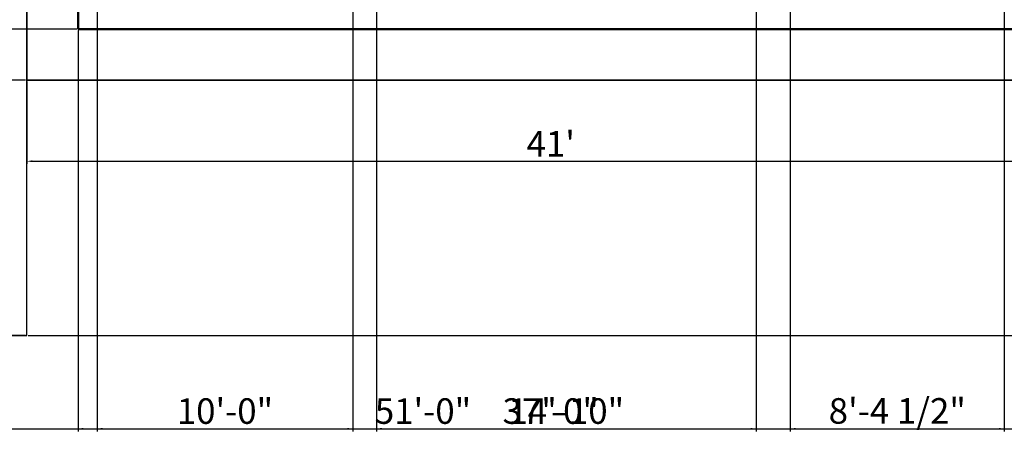
# Model space of a CAD drawing. Units: inches. Extents: x 5307 to 6359, y 4763 to 5474.
# Tile 2 of 5: x 5543 to 6006, y 4763 to 4966. Entities that reach past the tile are written whole.
import ezdxf

# ---------------------------------------------------------------- set-up
doc = ezdxf.new("R2010")
doc.units = ezdxf.units.IN
for name, color, linetype, lineweight in [('A-ANNO-DIMS', 2, 'Continuous', 18), ('A-WALL', 7, 'Continuous', 50), ('C-PROP', 7, 'Continuous', 35), ('ROAD', 240, 'Continuous', 25)]:
    doc.layers.add(name, color=color, linetype=linetype, lineweight=lineweight)
doc.styles.get("Standard").update_dxf_attribs({"font": 'arial.ttf'})
doc.dimstyles.new('ISO-25', dxfattribs={"dimtxt": 12, "dimasz": 2.5, "dimexe": 1.25, "dimexo": 0.625, "dimtad": 1, "dimtih": 1, "dimtoh": 1, "dimlunit": 4, "dimtxsty": 'Standard', "dimcen": 2.5, "dimadec": 0, "dimazin": 0, "dimtfac": 1, "dimtmove": 0, "dimatfit": 3, "dimfxl": 1, "dimarcsym": 0})

# ---------------------------------------------------------------- blocks, each defined once
blk = doc.blocks.new('*D3')
at = {"layer": 'A-ANNO-DIMS', "color": 0, "lineweight": -2, "transparency": 16777216}
for p, q in [((5545.97, 5237.78), (5511.45, 5237.78)), ((5512.7, 5235.28), (5512.7, 5094.54)), ((5512.7, 4940.28), (5512.7, 5081.03)), ((5545.97, 4937.78), (5511.45, 4937.78))]:
    blk.add_line(p, q, dxfattribs=at)
at = {"layer": 'A-ANNO-DIMS', "color": 0, "transparency": 16777216}
for points in [[(5512.28, 5235.28), (5513.12, 5235.28), (5512.7, 5237.78)], [(5512.28, 4940.28), (5513.12, 4940.28), (5512.7, 4937.78)]]:
    blk.add_solid(points, dxfattribs=at)
at = {"layer": 'Defpoints', "color": 0, "transparency": 16777216}
for p in [(5546.59, 5237.78), (5512.7, 4937.78), (5546.59, 4937.78)]:
    blk.add_point(p, dxfattribs=at)
at = {"layer": 'A-ANNO-DIMS', "color": 0, "transparency": 16777216, "insert": (5512.7, 5087.78), "char_height": 12, "attachment_point": 5}
blk.add_mtext("25'", dxfattribs=at)
blk = doc.blocks.new('*D4')
at = {"layer": 'A-ANNO-DIMS', "color": 0, "lineweight": -2, "transparency": 16777216}
for p, q in [((5546.59, 4937.16), (5546.59, 4898.47)), ((6038.59, 4937.64), (6038.59, 4898.47)), ((5549.09, 4899.72), (6036.09, 4899.72))]:
    blk.add_line(p, q, dxfattribs=at)
at = {"layer": 'A-ANNO-DIMS', "color": 0, "transparency": 16777216}
for points in [[(5549.09, 4900.14), (5549.09, 4899.3), (5546.59, 4899.72)], [(6036.09, 4900.14), (6036.09, 4899.3), (6038.59, 4899.72)]]:
    blk.add_solid(points, dxfattribs=at)
at = {"layer": 'Defpoints', "color": 0, "transparency": 16777216}
for p in [(6038.59, 4938.26), (5546.59, 4937.78), (6038.59, 4899.72)]:
    blk.add_point(p, dxfattribs=at)
at = {"layer": 'A-ANNO-DIMS', "color": 0, "transparency": 16777216, "insert": (5792.59, 4906.37), "char_height": 12, "attachment_point": 5}
blk.add_mtext("41'", dxfattribs=at)
blk = doc.blocks.new('*D12')
at = {"layer": 'A-ANNO-DIMS', "color": 0, "lineweight": -2, "transparency": 16777216}
for p, q in [((6038.59, 4937.16), (6038.59, 4772.78)), ((5426.59, 4817.16), (5426.59, 4772.78)), ((5429.09, 4774.03), (6036.09, 4774.03))]:
    blk.add_line(p, q, dxfattribs=at)
at = {"layer": 'A-ANNO-DIMS', "color": 0, "transparency": 16777216}
for points in [[(5429.09, 4774.45), (5429.09, 4773.62), (5426.59, 4774.03)], [(6036.09, 4774.45), (6036.09, 4773.62), (6038.59, 4774.03)]]:
    blk.add_solid(points, dxfattribs=at)
at = {"layer": 'Defpoints', "color": 0, "transparency": 16777216}
for p in [(6038.59, 4937.78), (5426.59, 4817.78), (6038.59, 4774.03)]:
    blk.add_point(p, dxfattribs=at)
at = {"layer": 'A-ANNO-DIMS', "color": 0, "transparency": 16777216, "insert": (5732.59, 4780.79), "char_height": 12, "attachment_point": 5}
blk.add_mtext('51\'-0"', dxfattribs=at)
blk = doc.blocks.new('*D13')
at = {"layer": 'A-ANNO-DIMS', "color": 0, "lineweight": -2, "transparency": 16777216}
for p, q in [((6038.88, 5405.78), (6325.25, 5405.78)), ((6324, 5403.28), (6324, 5118.54)), ((6324, 4820.28), (6324, 5105.03)), ((5547.22, 4817.78), (6325.25, 4817.78))]:
    blk.add_line(p, q, dxfattribs=at)
at = {"layer": 'A-ANNO-DIMS', "color": 0, "transparency": 16777216}
for points in [[(6323.58, 5403.28), (6324.41, 5403.28), (6324, 5405.78)], [(6323.58, 4820.28), (6324.41, 4820.28), (6324, 4817.78)]]:
    blk.add_solid(points, dxfattribs=at)
at = {"layer": 'Defpoints', "color": 0, "transparency": 16777216}
for p in [(6038.25, 5405.78), (6324, 5405.78), (5546.59, 4817.78)]:
    blk.add_point(p, dxfattribs=at)
at = {"layer": 'A-ANNO-DIMS', "color": 0, "transparency": 16777216, "insert": (6324, 5111.78), "char_height": 12, "attachment_point": 5}
blk.add_mtext('49\'-0"', dxfattribs=at)
blk = doc.blocks.new('*D15')
at = {"layer": 'A-ANNO-DIMS', "color": 0, "lineweight": -2, "transparency": 16777216}
for p, q in [((5569.97, 4961.78), (5381.59, 4961.78)), ((5382.84, 4959.28), (5382.84, 4956.54)), ((5382.84, 4940.28), (5382.84, 4943.03)), ((5545.97, 4937.78), (5381.59, 4937.78))]:
    blk.add_line(p, q, dxfattribs=at)
at = {"layer": 'A-ANNO-DIMS', "color": 0, "transparency": 16777216}
for points in [[(5382.43, 4959.28), (5383.26, 4959.28), (5382.84, 4961.78)], [(5382.43, 4940.28), (5383.26, 4940.28), (5382.84, 4937.78)]]:
    blk.add_solid(points, dxfattribs=at)
at = {"layer": 'Defpoints', "color": 0, "transparency": 16777216}
for p in [(5382.84, 4961.78), (5570.59, 4961.78), (5546.59, 4937.78)]:
    blk.add_point(p, dxfattribs=at)
at = {"layer": 'A-ANNO-DIMS', "color": 0, "transparency": 16777216, "insert": (5382.84, 4949.78), "char_height": 12, "attachment_point": 5}
blk.add_mtext('2\'-0"', dxfattribs=at)
blk = doc.blocks.new('*D18')
at = {"layer": 'A-ANNO-DIMS', "color": 0, "lineweight": -2, "transparency": 16777216}
for p, q in [((5545.97, 4937.78), (5381.59, 4937.78)), ((5382.84, 4935.28), (5382.84, 4884.54)), ((5382.84, 4820.28), (5382.84, 4871.03)), ((5545.97, 4817.78), (5381.59, 4817.78))]:
    blk.add_line(p, q, dxfattribs=at)
at = {"layer": 'A-ANNO-DIMS', "color": 0, "transparency": 16777216}
for points in [[(5382.43, 4935.28), (5383.26, 4935.28), (5382.84, 4937.78)], [(5382.43, 4820.28), (5383.26, 4820.28), (5382.84, 4817.78)]]:
    blk.add_solid(points, dxfattribs=at)
at = {"layer": 'Defpoints', "color": 0, "transparency": 16777216}
for p in [(5382.84, 4937.78), (5546.59, 4937.78), (5546.59, 4817.78)]:
    blk.add_point(p, dxfattribs=at)
at = {"layer": 'A-ANNO-DIMS', "color": 0, "transparency": 16777216, "insert": (5382.84, 4877.78), "char_height": 12, "attachment_point": 5}
blk.add_mtext('10\'-0"', dxfattribs=at)
blk = doc.blocks.new('*D24')
at = {"layer": 'A-ANNO-DIMS', "color": 0, "lineweight": -2, "transparency": 16777216}
for p, q in [((5579.59, 4970.16), (5579.59, 4772.78)), ((5699.59, 4970.16), (5699.59, 4772.78)), ((5582.09, 4774.03), (5697.09, 4774.03))]:
    blk.add_line(p, q, dxfattribs=at)
at = {"layer": 'A-ANNO-DIMS', "color": 0, "transparency": 16777216}
for points in [[(5582.09, 4774.45), (5582.09, 4773.62), (5579.59, 4774.03)], [(5697.09, 4774.45), (5697.09, 4773.62), (5699.59, 4774.03)]]:
    blk.add_solid(points, dxfattribs=at)
at = {"layer": 'Defpoints', "color": 0, "transparency": 16777216}
for p in [(5579.59, 4970.78), (5699.59, 4970.78), (5699.59, 4774.03)]:
    blk.add_point(p, dxfattribs=at)
at = {"layer": 'A-ANNO-DIMS', "color": 0, "transparency": 16777216, "insert": (5639.59, 4780.79), "char_height": 12, "attachment_point": 5}
blk.add_mtext('10\'-0"', dxfattribs=at)
blk = doc.blocks.new('*D25')
at = {"layer": 'A-ANNO-DIMS', "color": 0, "lineweight": -2, "transparency": 16777216}
for p, q in [((5710.76, 4970.16), (5710.76, 4772.78)), ((5889, 4970.05), (5889, 4772.78)), ((5713.26, 4774.03), (5886.5, 4774.03))]:
    blk.add_line(p, q, dxfattribs=at)
at = {"layer": 'A-ANNO-DIMS', "color": 0, "transparency": 16777216}
for points in [[(5713.26, 4774.45), (5713.26, 4773.62), (5710.76, 4774.03)], [(5886.5, 4774.45), (5886.5, 4773.62), (5889, 4774.03)]]:
    blk.add_solid(points, dxfattribs=at)
at = {"layer": 'Defpoints', "color": 0, "transparency": 16777216}
for p in [(5710.76, 4970.78), (5889, 4970.67), (5889, 4774.03)]:
    blk.add_point(p, dxfattribs=at)
at = {"layer": 'A-ANNO-DIMS', "color": 0, "transparency": 16777216, "insert": (5799.88, 4780.79), "char_height": 12, "attachment_point": 5}
blk.add_mtext('14\'-10"', dxfattribs=at)
blk = doc.blocks.new('*D26')
at = {"layer": 'A-ANNO-DIMS', "color": 0, "lineweight": -2, "transparency": 16777216}
for p, q in [((5905.06, 4970.06), (5905.06, 4772.78)), ((6005.56, 4970.16), (6005.56, 4772.78)), ((5907.56, 4774.03), (6003.06, 4774.03))]:
    blk.add_line(p, q, dxfattribs=at)
at = {"layer": 'A-ANNO-DIMS', "color": 0, "transparency": 16777216}
for points in [[(5907.56, 4774.45), (5907.56, 4773.62), (5905.06, 4774.03)], [(6003.06, 4774.45), (6003.06, 4773.62), (6005.56, 4774.03)]]:
    blk.add_solid(points, dxfattribs=at)
at = {"layer": 'Defpoints', "color": 0, "transparency": 16777216}
for p in [(5905.06, 4970.69), (6005.56, 4970.78), (6005.56, 4774.03)]:
    blk.add_point(p, dxfattribs=at)
at = {"layer": 'A-ANNO-DIMS', "color": 0, "transparency": 16777216, "insert": (5955.31, 4780.86), "char_height": 12, "attachment_point": 5}
blk.add_mtext('8\'-4 1/2"', dxfattribs=at)
blk = doc.blocks.new('*D33')
at = {"layer": 'A-ANNO-DIMS', "color": 0, "lineweight": -2, "transparency": 16777216}
for p, q in [((5570.59, 4961.16), (5570.59, 4772.78)), ((6014.57, 4961.16), (6014.57, 4772.78)), ((5573.09, 4774.03), (6012.07, 4774.03))]:
    blk.add_line(p, q, dxfattribs=at)
at = {"layer": 'A-ANNO-DIMS', "color": 0, "transparency": 16777216}
for points in [[(5573.09, 4774.45), (5573.09, 4773.62), (5570.59, 4774.03)], [(6012.07, 4774.45), (6012.07, 4773.62), (6014.57, 4774.03)]]:
    blk.add_solid(points, dxfattribs=at)
at = {"layer": 'Defpoints', "color": 0, "transparency": 16777216}
for p in [(5570.59, 4961.78), (6014.57, 4961.78), (6014.57, 4774.03)]:
    blk.add_point(p, dxfattribs=at)
at = {"layer": 'A-ANNO-DIMS', "color": 0, "transparency": 16777216, "insert": (5792.58, 4780.79), "char_height": 12, "attachment_point": 5}
blk.add_mtext('37\'-0"', dxfattribs=at)

msp = doc.modelspace()

# ---------------------------------------------------------------- linework, layer by layer
at = {"layer": 'A-WALL'}
for p, q in [((5570.592, 5213.807), (5570.592, 4961.784)), ((5570.592, 4961.784), (6014.569, 4961.784)), ((5881.069, 4961.654), (5881.069, 4961.784)), ((5885.569, 4961.659), (5885.569, 4961.784))]:
    msp.add_line(p, q, dxfattribs=at)
at = {"layer": 'C-PROP'}
for p, q in [((5546.592, 5237.784), (5546.592, 4937.784)), ((5546.592, 4937.784), (6038.592, 4937.784))]:
    msp.add_line(p, q, dxfattribs=at)
at = {"layer": 'ROAD'}
for p, q in [((5546.592, 4817.784), (5546.592, 4937.784)), ((5426.592, 4817.784), (5546.592, 4817.784))]:
    msp.add_line(p, q, dxfattribs=at)

# ---------------------------------------------------------------- dimensions: what is measured, and where the dimension line sits
at = {"layer": 'A-ANNO-DIMS'}
for base, p1, p2, override, picture, middle in [((6323.996, 5405.784), (5546.592, 4817.784), (6038.255, 5405.784), {"dimdec": 1, "dimlfac": 1, "dimrnd": 0, "dimzin": 1, "dimdsep": 46, "dimlunit": 4, "dimfrac": 2}, '*D13', (6323.996, 5111.784)), ((5512.7, 4937.784), (5546.592, 5237.784), (5546.592, 4937.784), {"dimclrd": 0, "dimclre": 0, "dimclrt": 0}, '*D3', (5512.7, 5087.784)), ((5382.842, 4961.784), (5546.592, 4937.784), (5570.592, 4961.784), {"dimdec": 1, "dimlfac": 1, "dimrnd": 0, "dimzin": 1, "dimdsep": 46, "dimlunit": 4, "dimfrac": 2}, '*D15', (5382.842, 4949.784)), ((5382.842, 4937.784), (5546.592, 4817.784), (5546.592, 4937.784), {"dimdec": 1, "dimlfac": 1, "dimrnd": 0, "dimzin": 1, "dimdsep": 46, "dimlunit": 4, "dimfrac": 2}, '*D18', (5382.842, 4877.784))]:
    dim = msp.add_linear_dim(base=base, p1=p1, p2=p2, angle=90, dimstyle='ISO-25', override=override, dxfattribs=at)
    dim.commit()
    dim.dimension.update_dxf_attribs({"geometry": picture, "text_midpoint": middle})
for base, p1, p2, override, picture, middle in [((5699.592, 4774.034), (5579.592, 4970.784), (5699.592, 4970.784), {"dimdec": 1, "dimlfac": 1, "dimrnd": 0, "dimzin": 1, "dimdsep": 46, "dimlunit": 4, "dimfrac": 2}, '*D24', (5639.592, 4780.786)), ((5889.001, 4774.034), (5710.758, 4970.784), (5889.001, 4970.671), {"dimdec": 1, "dimlfac": 1, "dimrnd": 0, "dimzin": 1, "dimdsep": 46, "dimlunit": 4, "dimfrac": 2}, '*D25', (5799.88, 4780.786)), ((6005.56, 4774.034), (5905.06, 4970.686), (6005.56, 4970.784), {"dimdec": 1, "dimlfac": 1, "dimrnd": 0, "dimzin": 1, "dimdsep": 46, "dimlunit": 4, "dimfrac": 2}, '*D26', (5955.31, 4780.864)), ((6014.569, 4774.034), (5570.592, 4961.784), (6014.569, 4961.784), {"dimdec": 1, "dimlfac": 1, "dimrnd": 0, "dimzin": 1, "dimdsep": 46, "dimlunit": 4, "dimfrac": 2}, '*D33', (5792.581, 4780.79)), ((6038.592, 4899.719), (5546.592, 4937.784), (6038.592, 4938.261), {"dimclrd": 0, "dimclre": 0, "dimclrt": 0}, '*D4', (5792.592, 4906.368)), ((6038.592, 4774.034), (5426.592, 4817.784), (6038.592, 4937.784), {"dimdec": 1, "dimlfac": 1, "dimrnd": 0, "dimzin": 1, "dimdsep": 46, "dimlunit": 4, "dimfrac": 2}, '*D12', (5732.592, 4780.786))]:
    dim = msp.add_linear_dim(base=base, p1=p1, p2=p2, dimstyle='ISO-25', override=override, dxfattribs=at)
    dim.commit()
    dim.dimension.update_dxf_attribs({"geometry": picture, "text_midpoint": middle})

doc.saveas('drawing.dxf')
